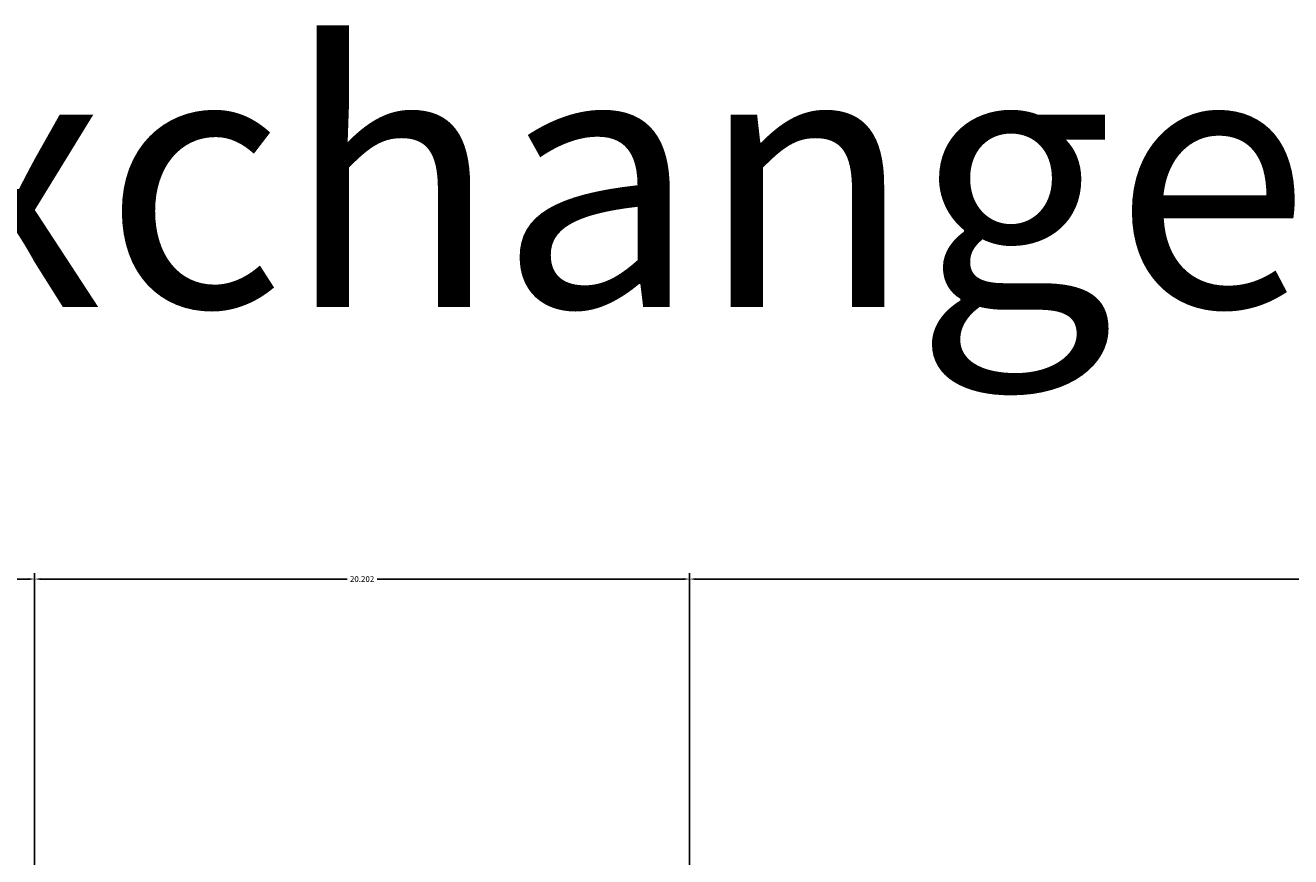
# Model space of a CAD drawing. Units: inches. Extents: x -12 to 334, y -10 to 186.
# Tile 61 of 77: x 106 to 145, y 161 to 186. Entities that reach past the tile are written whole.
import ezdxf

# ---------------------------------------------------------------- set-up
doc = ezdxf.new("R2010")
doc.units = ezdxf.units.IN
doc.header["$MEASUREMENT"] = 0
doc.layers.add('M-ANNO-TEXT', color=3, linetype='Continuous', lineweight=25)
doc.layers.add('M-DIMS', color=2, linetype='Continuous', lineweight=18)
doc.styles.get("Standard").update_dxf_attribs({"font": 'arial.ttf'})
doc.dimstyles.get("Standard").update_dxf_attribs({"dimtxt": 0.18, "dimasz": 0.18, "dimexe": 0.18, "dimexo": 0.0625, "dimgap": 0.09, "dimtad": 0, "dimtih": 1, "dimtoh": 1, "dimdec": 4, "dimzin": 0, "dimdsep": 46, "dimtxsty": 'Standard', "dimcen": 0.09, "dimadec": 0, "dimazin": 0, "dimtfac": 1, "dimtdec": 4, "dimtofl": 0, "dimtmove": 0, "dimatfit": 3, "dimfxl": 1, "dimtolj": 1, "dimtzin": 0, "dimarcsym": 0})

# ---------------------------------------------------------------- blocks, each defined once
blk = doc.blocks.new('*D15')
at = {"layer": 'Defpoints', "color": 0, "transparency": 16777216}
for p in [(106.177, 169.385), (86.888, 109.058), (106.177, 102.896)]:
    blk.add_point(p, dxfattribs=at)
at = {"layer": 'M-DIMS', "color": 0, "lineweight": -2, "transparency": 16777216}
for p, q in [((86.888, 109.121), (86.888, 169.565)), ((87.068, 169.385), (96.147, 169.385)), ((105.997, 169.385), (96.918, 169.385)), ((106.177, 102.958), (106.177, 169.565))]:
    blk.add_line(p, q, dxfattribs=at)
at = {"layer": 'M-DIMS', "color": 0, "transparency": 16777216}
for points in [[(87.068, 169.415), (87.068, 169.355), (86.888, 169.385)], [(105.997, 169.415), (105.997, 169.355), (106.177, 169.385)]]:
    blk.add_solid(points, dxfattribs=at)
at = {"layer": 'M-DIMS', "color": 0, "transparency": 16777216, "insert": (96.532, 169.385), "char_height": 0.18, "attachment_point": 5}
blk.add_mtext('\\A1;19.29', dxfattribs=at)
blk = doc.blocks.new('*D16')
at = {"layer": 'Defpoints', "color": 0, "transparency": 16777216}
for p in [(126.379, 169.385), (126.379, 137.887), (106.177, 102.896)]:
    blk.add_point(p, dxfattribs=at)
at = {"layer": 'M-DIMS', "color": 0, "lineweight": -2, "transparency": 16777216}
for p, q in [((106.177, 102.958), (106.177, 169.565)), ((106.357, 169.385), (115.814, 169.385)), ((126.199, 169.385), (116.742, 169.385)), ((126.379, 137.95), (126.379, 169.565))]:
    blk.add_line(p, q, dxfattribs=at)
at = {"layer": 'M-DIMS', "color": 0, "transparency": 16777216}
for points in [[(106.357, 169.415), (106.357, 169.355), (106.177, 169.385)], [(126.199, 169.415), (126.199, 169.355), (126.379, 169.385)]]:
    blk.add_solid(points, dxfattribs=at)
at = {"layer": 'M-DIMS', "color": 0, "transparency": 16777216, "insert": (116.278, 169.385), "char_height": 0.18, "attachment_point": 5}
blk.add_mtext('\\A1;20.202', dxfattribs=at)
blk = doc.blocks.new('*D18')
at = {"layer": 'Defpoints', "color": 0, "transparency": 16777216}
for p in [(190.342, 169.385), (190.342, 154.835), (126.379, 137.887)]:
    blk.add_point(p, dxfattribs=at)
at = {"layer": 'M-DIMS', "color": 0, "lineweight": -2, "transparency": 16777216}
for p, q in [((126.379, 137.95), (126.379, 169.565)), ((126.559, 169.385), (157.967, 169.385)), ((190.162, 169.385), (158.755, 169.385)), ((190.342, 154.897), (190.342, 169.565))]:
    blk.add_line(p, q, dxfattribs=at)
at = {"layer": 'M-DIMS', "color": 0, "transparency": 16777216}
for points in [[(126.559, 169.415), (126.559, 169.355), (126.379, 169.385)], [(190.162, 169.415), (190.162, 169.355), (190.342, 169.385)]]:
    blk.add_solid(points, dxfattribs=at)
at = {"layer": 'M-DIMS', "color": 0, "transparency": 16777216, "insert": (158.361, 169.385), "char_height": 0.18, "attachment_point": 5}
blk.add_mtext('\\A1;63.96', dxfattribs=at)

msp = doc.modelspace()

# ---------------------------------------------------------------- texts
at = {"layer": 'M-ANNO-TEXT', "insert": (70.1252, 185.7805), "char_height": 8, "attachment_point": 1}
msp.add_mtext_dynamic_manual_height_columns('Heat exchanger in a steam boiler', width=205.597506, gutter_width=1, heights=[0], dxfattribs=at)

# ---------------------------------------------------------------- dimensions: what is measured, and where the dimension line sits
at = {"layer": 'M-DIMS'}
for base, p1, p2, override, picture, middle in [((106.1771, 169.3845), (86.8879, 109.0583), (106.1771, 102.8958), {"dimdec": 2, "dimlfac": 1, "dimrnd": 0, "dimzin": 0, "dimdsep": 46, "dimlunit": 2}, '*D15', (96.5325, 169.3845)), ((126.3793, 169.3845), (106.1771, 102.8958), (126.3793, 137.8871), {"dimdec": 3, "dimlfac": 1, "dimrnd": 0, "dimzin": 0, "dimdsep": 46, "dimlunit": 2}, '*D16', (116.2782, 169.3845)), ((190.3421, 169.3845), (126.3793, 137.8871), (190.3421, 154.8345), {"dimdec": 2, "dimlfac": 1, "dimrnd": 0, "dimzin": 0, "dimdsep": 46, "dimlunit": 2}, '*D18', (158.3607, 169.3845))]:
    dim = msp.add_linear_dim(base=base, p1=p1, p2=p2, dimstyle='Standard', override=override, dxfattribs=at)
    dim.commit()
    dim.dimension.update_dxf_attribs({"geometry": picture, "text_midpoint": middle})

doc.saveas('drawing.dxf')
